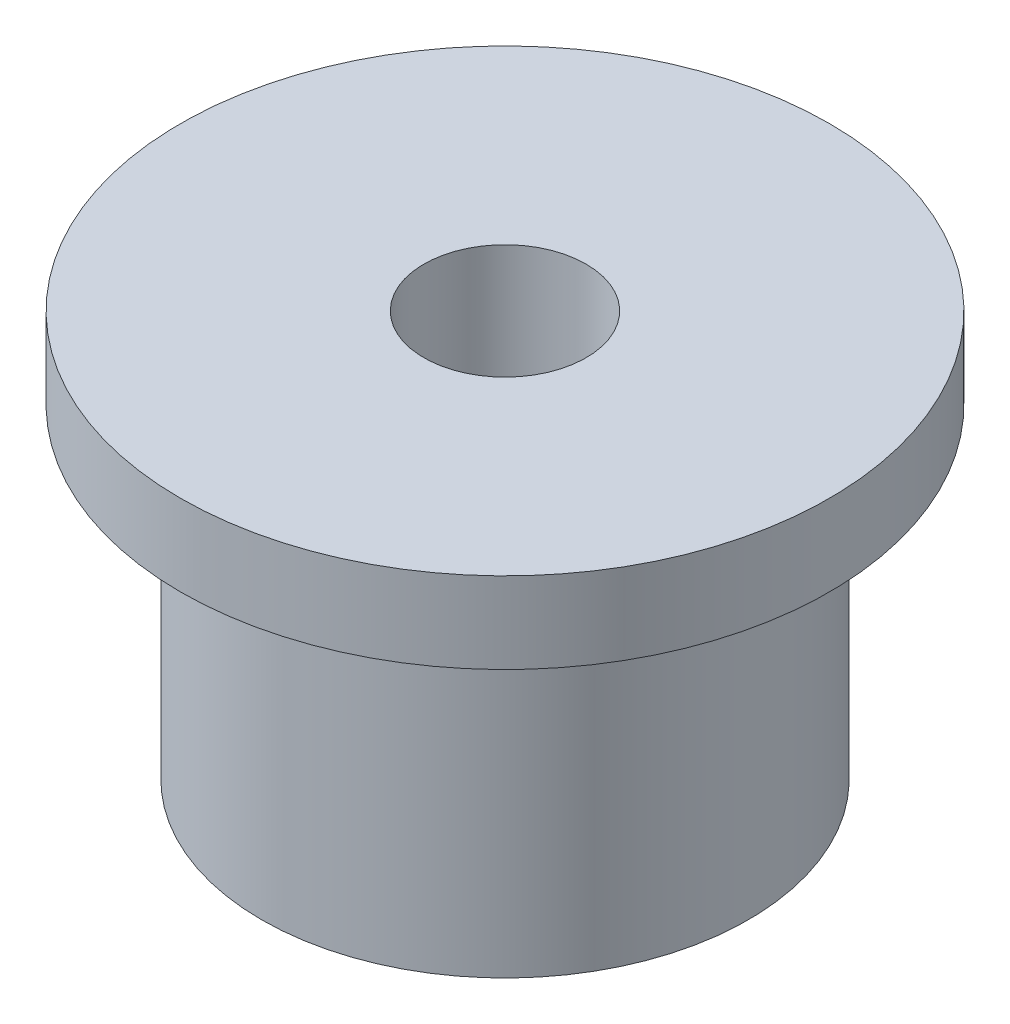
ISO-10303-21;
HEADER;
FILE_DESCRIPTION(('STEP AP214'),'2;1');
FILE_NAME('part.step','',(''),(''),'','','');
FILE_SCHEMA(('AUTOMOTIVE_DESIGN { 1 0 10303 214 1 1 1 1 }'));
ENDSEC;
DATA;
#1=APPLICATION_CONTEXT('core data for automotive mechanical design processes');
#2=APPLICATION_PROTOCOL_DEFINITION('international standard','automotive_design',2000,#1);
#3=PRODUCT_CONTEXT('',#1,'mechanical');
#4=PRODUCT('Part','Part','',(#3));
#5=PRODUCT_RELATED_PRODUCT_CATEGORY('part','',(#4));
#6=PRODUCT_DEFINITION_FORMATION('','',#4);
#7=PRODUCT_DEFINITION_CONTEXT('part definition',#1,'design');
#8=PRODUCT_DEFINITION('design','',#6,#7);
#9=PRODUCT_DEFINITION_SHAPE('','',#8);
#10=(LENGTH_UNIT() NAMED_UNIT(*) SI_UNIT(.MILLI.,.METRE.));
#11=(NAMED_UNIT(*) PLANE_ANGLE_UNIT() SI_UNIT($,.RADIAN.));
#12=(NAMED_UNIT(*) SI_UNIT($,.STERADIAN.) SOLID_ANGLE_UNIT());
#13=UNCERTAINTY_MEASURE_WITH_UNIT(LENGTH_MEASURE(1.E-05),#10,'distance_accuracy_value','');
#14=(GEOMETRIC_REPRESENTATION_CONTEXT(3) GLOBAL_UNCERTAINTY_ASSIGNED_CONTEXT((#13)) GLOBAL_UNIT_ASSIGNED_CONTEXT((#10,
#11,#12)) REPRESENTATION_CONTEXT('',''));
#15=CARTESIAN_POINT('',(0.,0.,0.));
#16=DIRECTION('',(0.,0.,1.));
#17=DIRECTION('',(1.,0.,0.));
#18=AXIS2_PLACEMENT_3D('',#15,#16,#17);
#19=CARTESIAN_POINT('',(75.,0.,0.));
#20=DIRECTION('',(0.,-1.,0.));
#21=DIRECTION('',(0.,0.,-1.));
#22=AXIS2_PLACEMENT_3D('',#19,#20,#21);
#23=PLANE('',#22);
#24=CARTESIAN_POINT('',(0.,0.,0.));
#25=DIRECTION('',(0.,-1.,0.));
#26=DIRECTION('',(0.,0.,-1.));
#27=AXIS2_PLACEMENT_3D('',#24,#25,#26);
#28=CIRCLE('',#27,75.);
#29=CARTESIAN_POINT('',(0.,0.,-75.));
#30=VERTEX_POINT('',#29);
#31=EDGE_CURVE('E56',#30,#30,#28,.T.);
#32=ORIENTED_EDGE('',*,*,#31,.T.);
#33=EDGE_LOOP('',(#32));
#34=FACE_BOUND('',#33,.T.);
#35=CARTESIAN_POINT('',(0.,0.,0.));
#36=DIRECTION('',(0.,-1.,0.));
#37=DIRECTION('',(0.,0.,-1.));
#38=AXIS2_PLACEMENT_3D('',#35,#36,#37);
#39=CIRCLE('',#38,25.);
#40=CARTESIAN_POINT('',(0.,0.,-25.));
#41=VERTEX_POINT('',#40);
#42=EDGE_CURVE('E10',#41,#41,#39,.T.);
#43=ORIENTED_EDGE('',*,*,#42,.F.);
#44=EDGE_LOOP('',(#43));
#45=FACE_BOUND('',#44,.T.);
#46=ADVANCED_FACE('F40',(#34,#45),#23,.T.);
#47=CARTESIAN_POINT('',(0.,0.,0.));
#48=DIRECTION('',(0.,-1.,0.));
#49=DIRECTION('',(0.,0.,-1.));
#50=AXIS2_PLACEMENT_3D('',#47,#48,#49);
#51=CYLINDRICAL_SURFACE('',#50,25.);
#52=ORIENTED_EDGE('',*,*,#42,.T.);
#53=EDGE_LOOP('',(#52));
#54=FACE_BOUND('',#53,.T.);
#55=CARTESIAN_POINT('',(0.,125.,0.));
#56=DIRECTION('',(0.,-1.,0.));
#57=DIRECTION('',(0.,0.,-1.));
#58=AXIS2_PLACEMENT_3D('',#55,#56,#57);
#59=CIRCLE('',#58,25.);
#60=CARTESIAN_POINT('',(0.,125.,-25.));
#61=VERTEX_POINT('',#60);
#62=EDGE_CURVE('E43',#61,#61,#59,.T.);
#63=ORIENTED_EDGE('',*,*,#62,.F.);
#64=EDGE_LOOP('',(#63));
#65=FACE_BOUND('',#64,.T.);
#66=ADVANCED_FACE('F80',(#54,#65),#51,.F.);
#67=CARTESIAN_POINT('',(25.,125.,0.));
#68=DIRECTION('',(0.,1.,0.));
#69=DIRECTION('',(0.,0.,1.));
#70=AXIS2_PLACEMENT_3D('',#67,#68,#69);
#71=PLANE('',#70);
#72=ORIENTED_EDGE('',*,*,#62,.T.);
#73=EDGE_LOOP('',(#72));
#74=FACE_BOUND('',#73,.T.);
#75=CARTESIAN_POINT('',(0.,125.,0.));
#76=DIRECTION('',(0.,-1.,0.));
#77=DIRECTION('',(0.,0.,-1.));
#78=AXIS2_PLACEMENT_3D('',#75,#76,#77);
#79=CIRCLE('',#78,100.);
#80=CARTESIAN_POINT('',(0.,125.,-100.));
#81=VERTEX_POINT('',#80);
#82=EDGE_CURVE('E50',#81,#81,#79,.T.);
#83=ORIENTED_EDGE('',*,*,#82,.F.);
#84=EDGE_LOOP('',(#83));
#85=FACE_BOUND('',#84,.T.);
#86=ADVANCED_FACE('F83',(#74,#85),#71,.T.);
#87=CARTESIAN_POINT('',(0.,0.,0.));
#88=DIRECTION('',(0.,-1.,0.));
#89=DIRECTION('',(0.,0.,-1.));
#90=AXIS2_PLACEMENT_3D('',#87,#88,#89);
#91=CYLINDRICAL_SURFACE('',#90,100.);
#92=ORIENTED_EDGE('',*,*,#82,.T.);
#93=EDGE_LOOP('',(#92));
#94=FACE_BOUND('',#93,.T.);
#95=CARTESIAN_POINT('',(0.,100.,0.));
#96=DIRECTION('',(0.,-1.,0.));
#97=DIRECTION('',(0.,0.,-1.));
#98=AXIS2_PLACEMENT_3D('',#95,#96,#97);
#99=CIRCLE('',#98,100.);
#100=CARTESIAN_POINT('',(0.,100.,-100.));
#101=VERTEX_POINT('',#100);
#102=EDGE_CURVE('E51',#101,#101,#99,.T.);
#103=ORIENTED_EDGE('',*,*,#102,.F.);
#104=EDGE_LOOP('',(#103));
#105=FACE_BOUND('',#104,.T.);
#106=ADVANCED_FACE('F71',(#94,#105),#91,.T.);
#107=CARTESIAN_POINT('',(100.,100.,0.));
#108=DIRECTION('',(0.,-1.,0.));
#109=DIRECTION('',(0.,0.,-1.));
#110=AXIS2_PLACEMENT_3D('',#107,#108,#109);
#111=PLANE('',#110);
#112=ORIENTED_EDGE('',*,*,#102,.T.);
#113=EDGE_LOOP('',(#112));
#114=FACE_BOUND('',#113,.T.);
#115=CARTESIAN_POINT('',(0.,100.,0.));
#116=DIRECTION('',(0.,-1.,0.));
#117=DIRECTION('',(0.,0.,-1.));
#118=AXIS2_PLACEMENT_3D('',#115,#116,#117);
#119=CIRCLE('',#118,75.);
#120=CARTESIAN_POINT('',(0.,100.,-75.));
#121=VERTEX_POINT('',#120);
#122=EDGE_CURVE('E57',#121,#121,#119,.T.);
#123=ORIENTED_EDGE('',*,*,#122,.F.);
#124=EDGE_LOOP('',(#123));
#125=FACE_BOUND('',#124,.T.);
#126=ADVANCED_FACE('F70',(#114,#125),#111,.T.);
#127=CARTESIAN_POINT('',(0.,0.,0.));
#128=DIRECTION('',(0.,-1.,0.));
#129=DIRECTION('',(0.,0.,-1.));
#130=AXIS2_PLACEMENT_3D('',#127,#128,#129);
#131=CYLINDRICAL_SURFACE('',#130,75.);
#132=ORIENTED_EDGE('',*,*,#122,.T.);
#133=EDGE_LOOP('',(#132));
#134=FACE_BOUND('',#133,.T.);
#135=ORIENTED_EDGE('',*,*,#31,.F.);
#136=EDGE_LOOP('',(#135));
#137=FACE_BOUND('',#136,.T.);
#138=ADVANCED_FACE('F63',(#134,#137),#131,.T.);
#139=CLOSED_SHELL('',(#46,#66,#86,#106,#126,#138));
#140=MANIFOLD_SOLID_BREP('B2',#139);
#141=ADVANCED_BREP_SHAPE_REPRESENTATION('',(#18,#140),#14);
#142=SHAPE_DEFINITION_REPRESENTATION(#9,#141);
ENDSEC;
END-ISO-10303-21;
